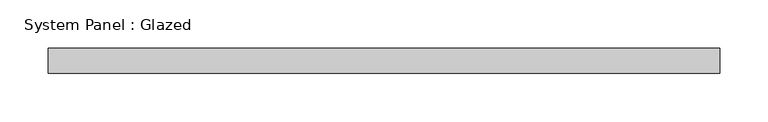
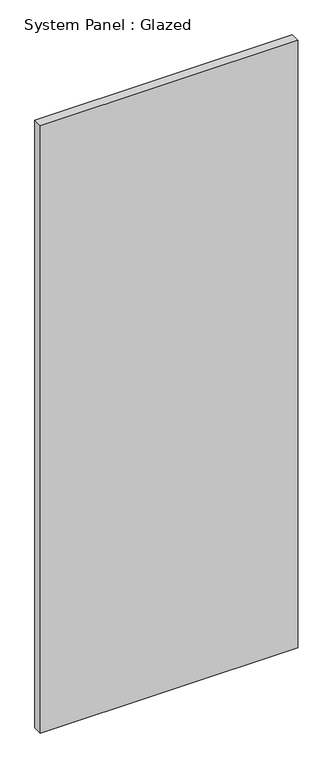
"""IFC4 building model written with IfcOpenShell, lengths in millimetres: plate geometry, System Panel : Glazed."""

from ifc_helpers import new_model, si_unit, origin, origin_with_axes, place, context, project, spatial, polyline, outline, extrude, source, transform, mapped, element, save


def system_panel_glazed_8f71a385(model_context):
    return source(origin(), model_context, "Body", "SweptSolid", [
        extrude(outline(polyline([(346.075, 19.05), (-346.075, 19.05), (-346.075, 44.45), (346.075, 44.45), (346.075, 19.05)])), origin_with_axes(), (0.0, 0.0, 1.0), 1725.7814546),
    ])


if __name__ == "__main__":
    model = new_model("IFC4")
    model_context = context("Model", 3, world=origin())
    ifc_project = project(units=[si_unit("LENGTHUNIT", "METRE", prefix="MILLI")], contexts=[model_context])
    site = spatial("IfcSite", under=ifc_project)
    building = spatial("IfcBuilding", under=site)
    placement = place(None, origin())
    system_panel_glazed_shape = system_panel_glazed_8f71a385(model_context)
    element("IfcPlate", 1, ObjectType="System Panel : Glazed", at=placement, inside=building, context=model_context, shape_type="MappedRepresentation", body=[
        mapped(system_panel_glazed_shape, transform((0.0, 0.0, 0.0), x_axis=(1.0, 0.0, 0.0), y_axis=(0.0, 1.0, 0.0), z_axis=(0.0, 0.0, 1.0))),
    ])
    save(model, "model.ifc")

# Revit data of these elements
# Type "System Panel : Glazed"
#   Construction Type Id = "GSP4R"
#   Analytic Construction = "1/8 in Pilkington single glazing"
#   Visual Light Transmittance = 0.9
#   Solar Heat Gain Coefficient = 0.86
#   Heat Transfer Coefficient (U) = 1.18115 BTU/(h·ft²·°F)
#   Define Thermal Properties by = 1
# Element 1 (IfcPlate, "System Panel : Glazed")
#   Materials on its faces: "Glass"
# Materials
#   "Glass": class "Glass", colour RGB 0 128 192, transparency 0.75, Description = "Soda Lime Glass", Cost = 0
